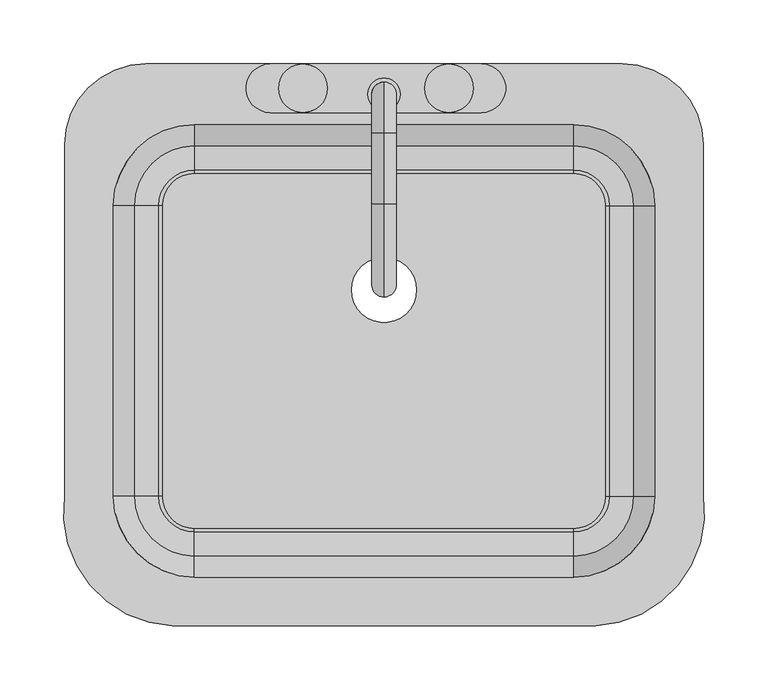
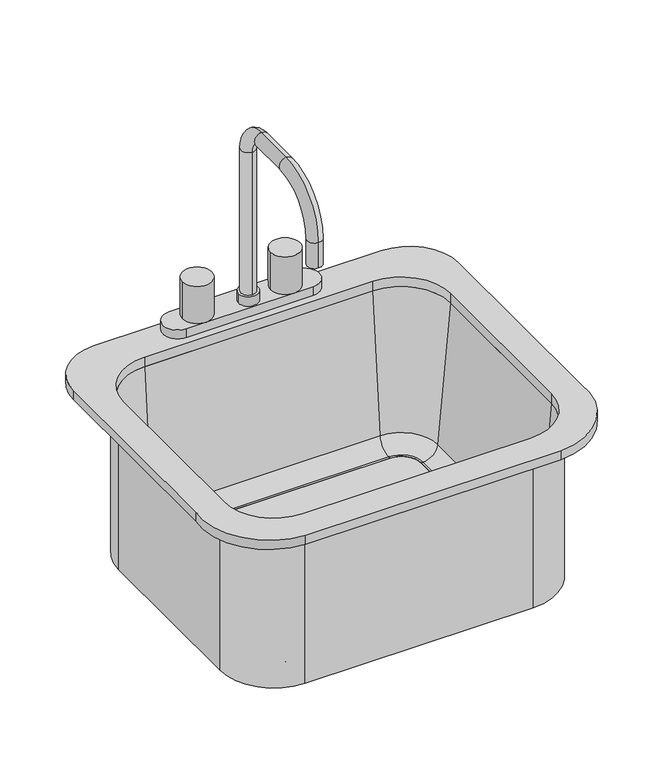
"""IFC4 building model written with IfcOpenShell, lengths in millimetres: flow terminal geometry."""

from ifc_helpers import new_model, si_unit, point, frame, frame_2d, origin, place, context, project, spatial, polyline, circle_curve, ellipse_curve, trimmed, segment, composite_curve, outline, extrude, source, transform, mapped, element, save
from ifc_brep_helpers import plane_surface, cylinder_surface, revolved_surface, advanced_brep


def flow_terminal_f629513f(model_context):
    return source(origin(), model_context, "Body", "SolidModel", [
        extrude(outline(composite_curve([segment(trimmed(circle_curve(frame_2d((-146.1534746, -170.8793432)), 89.0566732), [point((-149.9606923, -259.8545989))], [point((-234.3107593, -158.2545982))], False, "CARTESIAN"), True, "CONTINUOUS"), segment(polyline([(-234.3107593, -158.2545982), (-234.3107593, 116.6454011)]), True, "CONTINUOUS"), segment(trimmed(circle_curve(frame_2d((-170.8107593, 116.6454011)), 63.5), [point((-234.3107593, 116.6454011))], [point((-170.8107593, 180.1454011))], False, "CARTESIAN"), True, "CONTINUOUS"), segment(polyline([(-170.8107593, 180.1454011), (202.1892406, 180.1454011)]), True, "CONTINUOUS"), segment(trimmed(circle_curve(frame_2d((202.1892406, 116.6454011)), 63.5), [point((202.1892406, 180.1454011))], [point((265.6892406, 116.6454011))], False, "CARTESIAN"), True, "CONTINUOUS"), segment(polyline([(265.6892406, 116.6454011), (265.6892406, -158.2545989)]), True, "CONTINUOUS"), segment(trimmed(circle_curve(frame_2d((177.5319557, -170.8793432)), 89.0566732), [point((265.6892406, -158.2545989))], [point((181.3391735, -259.8545989))], False, "CARTESIAN"), True, "CONTINUOUS"), segment(polyline([(181.3391735, -259.8545989), (-149.9606923, -259.8545989)]), True, "CONTINUOUS")], self_intersect=False), holes=[composite_curve([segment(polyline([(164.0892406, 132.5204011), (-132.7107594, 132.5204011)]), True, "CONTINUOUS"), segment(trimmed(circle_curve(frame_2d((-132.7107594, 69.0204011)), 63.5), [point((-132.7107594, 132.5204011))], [point((-196.2107594, 69.0204011))], True, "CARTESIAN"), True, "CONTINUOUS"), segment(polyline([(-196.2107594, 69.0204011), (-196.2107594, -158.2545989)]), True, "CONTINUOUS"), segment(trimmed(circle_curve(frame_2d((-132.7107594, -158.2545989)), 63.5), [point((-196.2107594, -158.2545989))], [point((-132.7107594, -221.7545989))], True, "CARTESIAN"), True, "CONTINUOUS"), segment(polyline([(-132.7107594, -221.7545989), (164.0892406, -221.7545989)]), True, "CONTINUOUS"), segment(trimmed(circle_curve(frame_2d((164.0892406, -158.2545989)), 63.5), [point((164.0892406, -221.7545989))], [point((227.5892406, -158.2545989))], True, "CARTESIAN"), True, "CONTINUOUS"), segment(polyline([(227.5892406, -158.2545989), (227.5892406, 69.0204011)]), True, "CONTINUOUS"), segment(trimmed(circle_curve(frame_2d((164.0892406, 69.0204011)), 63.5), [point((227.5892406, 69.0204011))], [point((164.0892406, 132.5204011))], True, "CARTESIAN"), True, "CONTINUOUS")], self_intersect=False)]), frame((0.0, 0.0, 750.0), z_axis=(0.0, 0.0, 1.0), x_axis=(1.0, 0.0, 0.0)), (0.0, 0.0, 1.0), 12.7),
        advanced_brep(
        [(233.9392406, 69.0204011, 534.1), (164.0892406, 138.8704011, 534.1), (164.0892406, 138.8704011, 750.0), (233.9392406, 69.0204011, 750.0), (189.4892406, 69.0204011, 534.1), (164.0892406, 94.4204011, 534.1), (189.4892406, 69.0204011, 543.625), (164.0892406, 94.4204011, 543.625), (192.0776588, 69.0204011, 543.625), (164.0892406, 97.0088193, 543.625), (211.0551678, 69.0204011, 561.0146831), (164.0892406, 115.9863283, 561.0146831), (227.5892406, 69.0204011, 750.0), (164.0892406, 132.5204011, 750.0), (233.9392406, -158.2545989, 750.0), (233.9392406, -158.2545989, 534.1), (189.4892406, -158.2545989, 534.1), (189.4892406, -158.2545989, 543.625), (192.0776588, -158.2545989, 543.625), (211.0551678, -158.2545989, 561.0146831), (227.5892406, -158.2545989, 750.0), (164.0892406, -228.1045989, 534.1), (164.0892406, -228.1045989, 750.0), (164.0892406, -183.6545989, 534.1), (164.0892406, -183.6545989, 543.625), (164.0892406, -186.2430171, 543.625), (164.0892406, -205.2205261, 561.0146831), (164.0892406, -221.7545989, 750.0), (-132.7107594, -228.1045989, 750.0), (-132.7107594, -228.1045989, 534.1), (-132.7107594, -183.6545989, 534.1), (-132.7107594, -183.6545989, 543.625), (-132.7107594, -186.2430171, 543.625), (-132.7107594, -205.2205261, 561.0146831), (-132.7107594, -221.7545989, 750.0), (-202.5607594, -158.2545989, 534.1), (-202.5607594, -158.2545989, 750.0), (-158.1107594, -158.2545989, 534.1), (-158.1107594, -158.2545989, 543.625), (-160.6991776, -158.2545989, 543.625), (-179.6766866, -158.2545989, 561.0146831), (-196.2107594, -158.2545989, 750.0), (-202.5607594, 69.0204011, 750.0), (-202.5607594, 69.0204011, 534.1), (-158.1107594, 69.0204011, 534.1), (-158.1107594, 69.0204011, 543.625), (-160.6991776, 69.0204011, 543.625), (-179.6766866, 69.0204011, 561.0146831), (-196.2107594, 69.0204011, 750.0), (-132.7107594, 138.8704011, 534.1), (-132.7107594, 138.8704011, 750.0), (-132.7107594, 94.4204011, 534.1), (-132.7107594, 94.4204011, 543.625), (-132.7107594, 97.0088193, 543.625), (-132.7107594, 115.9863283, 561.0146831), (-132.7107594, 132.5204011, 750.0)],
        [
            (0, 1, circle_curve(frame((164.0892406, 69.0204011, 534.1), z_axis=(0.0, 0.0, 1.0), x_axis=(0.0, 1.0, 0.0)), 69.85)),
            (1, 2),
            (2, 3, circle_curve(frame((164.0892406, 69.0204011, 750.0), z_axis=(0.0, 0.0, -1.0), x_axis=(0.0, 1.0, 0.0)), 69.85)),
            (3, 0),
            (4, 5, circle_curve(frame((164.0892406, 69.0204011, 534.1), z_axis=(0.0, 0.0, 1.0), x_axis=(0.0, 1.0, 0.0)), 25.4)),
            (5, 1),
            (0, 4),
            (6, 7, circle_curve(frame((164.0892406, 69.0204011, 543.625), z_axis=(0.0, 0.0, 1.0), x_axis=(0.0, 1.0, 0.0)), 25.4)),
            (7, 5),
            (4, 6),
            (8, 9, circle_curve(frame((164.0892406, 69.0204011, 543.625), z_axis=(0.0, 0.0, 1.0), x_axis=(0.0, 1.0, 0.0)), 27.9884182)),
            (9, 7),
            (6, 8),
            (10, 11, circle_curve(frame((164.0892406, 69.0204011, 561.0146831), z_axis=(0.0, 0.0, 1.0), x_axis=(0.0, 1.0, 0.0)), 46.9659272)),
            (11, 9, circle_curve(frame((164.0892406, 97.0088193, 562.675), z_axis=(-1.0, 0.0, 0.0), x_axis=(0.0, 1.0, 0.0)), 19.05)),
            (8, 10, circle_curve(frame((192.0776588, 69.0204011, 562.675), z_axis=(0.0, -1.0, 0.0), x_axis=(1.0, 0.0, 0.0)), 19.05)),
            (12, 13, circle_curve(frame((164.0892406, 69.0204011, 750.0), z_axis=(0.0, 0.0, 1.0), x_axis=(0.0, 1.0, 0.0)), 63.5)),
            (13, 11),
            (10, 12),
            (2, 13),
            (12, 3),
            (3, 14),
            (14, 15),
            (15, 0),
            (15, 16),
            (16, 4),
            (16, 17),
            (17, 6),
            (17, 18),
            (18, 8),
            (18, 19, circle_curve(frame((192.0776588, -158.2545989, 562.675), z_axis=(0.0, -1.0, 0.0), x_axis=(1.0, 0.0, 0.0)), 19.05)),
            (19, 10),
            (19, 20),
            (20, 12),
            (20, 14),
            (21, 15, circle_curve(frame((164.0892406, -158.2545989, 534.1), z_axis=(0.0, 0.0, 1.0), x_axis=(1.0, 0.0, 0.0)), 69.85)),
            (14, 22, circle_curve(frame((164.0892406, -158.2545989, 750.0), z_axis=(0.0, 0.0, -1.0), x_axis=(1.0, 0.0, 0.0)), 69.85)),
            (22, 21),
            (23, 16, circle_curve(frame((164.0892406, -158.2545989, 534.1), z_axis=(0.0, 0.0, 1.0), x_axis=(1.0, 0.0, 0.0)), 25.4)),
            (21, 23),
            (24, 17, circle_curve(frame((164.0892406, -158.2545989, 543.625), z_axis=(0.0, 0.0, 1.0), x_axis=(1.0, 0.0, 0.0)), 25.4)),
            (23, 24),
            (25, 18, circle_curve(frame((164.0892406, -158.2545989, 543.625), z_axis=(0.0, 0.0, 1.0), x_axis=(1.0, 0.0, 0.0)), 27.9884182)),
            (24, 25),
            (26, 19, circle_curve(frame((164.0892406, -158.2545989, 561.0146831), z_axis=(0.0, 0.0, 1.0), x_axis=(1.0, 0.0, 0.0)), 46.9659272)),
            (25, 26, circle_curve(frame((164.0892406, -186.2430171, 562.675), z_axis=(-1.0, 0.0, 0.0), x_axis=(0.0, -1.0, 0.0)), 19.05)),
            (27, 20, circle_curve(frame((164.0892406, -158.2545989, 750.0), z_axis=(0.0, 0.0, 1.0), x_axis=(1.0, 0.0, 0.0)), 63.5)),
            (26, 27),
            (27, 22),
            (22, 28),
            (28, 29),
            (29, 21),
            (29, 30),
            (30, 23),
            (30, 31),
            (31, 24),
            (31, 32),
            (32, 25),
            (32, 33, circle_curve(frame((-132.7107594, -186.2430171, 562.675), z_axis=(-1.0, 0.0, 0.0), x_axis=(0.0, -1.0, 0.0)), 19.05)),
            (33, 26),
            (33, 34),
            (34, 27),
            (34, 28),
            (35, 29, circle_curve(frame((-132.7107594, -158.2545989, 534.1), z_axis=(0.0, 0.0, 1.0), x_axis=(0.0, -1.0, 0.0)), 69.85)),
            (28, 36, circle_curve(frame((-132.7107594, -158.2545989, 750.0), z_axis=(0.0, 0.0, -1.0), x_axis=(0.0, -1.0, 0.0)), 69.85)),
            (36, 35),
            (37, 30, circle_curve(frame((-132.7107594, -158.2545989, 534.1), z_axis=(0.0, 0.0, 1.0), x_axis=(0.0, -1.0, 0.0)), 25.4)),
            (35, 37),
            (38, 31, circle_curve(frame((-132.7107594, -158.2545989, 543.625), z_axis=(0.0, 0.0, 1.0), x_axis=(0.0, -1.0, 0.0)), 25.4)),
            (37, 38),
            (39, 32, circle_curve(frame((-132.7107594, -158.2545989, 543.625), z_axis=(0.0, 0.0, 1.0), x_axis=(0.0, -1.0, 0.0)), 27.9884182)),
            (38, 39),
            (40, 33, circle_curve(frame((-132.7107594, -158.2545989, 561.0146831), z_axis=(0.0, 0.0, 1.0), x_axis=(0.0, -1.0, 0.0)), 46.9659272)),
            (39, 40, circle_curve(frame((-160.6991776, -158.2545989, 562.675), z_axis=(0.0, 1.0, 0.0), x_axis=(-1.0, 0.0, 0.0)), 19.05)),
            (41, 34, circle_curve(frame((-132.7107594, -158.2545989, 750.0), z_axis=(0.0, 0.0, 1.0), x_axis=(0.0, -1.0, 0.0)), 63.5)),
            (40, 41),
            (41, 36),
            (36, 42),
            (42, 43),
            (43, 35),
            (43, 44),
            (44, 37),
            (44, 45),
            (45, 38),
            (45, 46),
            (46, 39),
            (46, 47, circle_curve(frame((-160.6991776, 69.0204011, 562.675), z_axis=(0.0, 1.0, 0.0), x_axis=(-1.0, 0.0, 0.0)), 19.05)),
            (47, 40),
            (47, 48),
            (48, 41),
            (48, 42),
            (49, 43, circle_curve(frame((-132.7107594, 69.0204011, 534.1), z_axis=(0.0, 0.0, 1.0), x_axis=(-1.0, 0.0, 0.0)), 69.85)),
            (42, 50, circle_curve(frame((-132.7107594, 69.0204011, 750.0), z_axis=(0.0, 0.0, -1.0), x_axis=(-1.0, 0.0, 0.0)), 69.85)),
            (50, 49),
            (51, 44, circle_curve(frame((-132.7107594, 69.0204011, 534.1), z_axis=(0.0, 0.0, 1.0), x_axis=(-1.0, 0.0, 0.0)), 25.4)),
            (49, 51),
            (52, 45, circle_curve(frame((-132.7107594, 69.0204011, 543.625), z_axis=(0.0, 0.0, 1.0), x_axis=(-1.0, 0.0, 0.0)), 25.4)),
            (51, 52),
            (53, 46, circle_curve(frame((-132.7107594, 69.0204011, 543.625), z_axis=(0.0, 0.0, 1.0), x_axis=(-1.0, 0.0, 0.0)), 27.9884182)),
            (52, 53),
            (54, 47, circle_curve(frame((-132.7107594, 69.0204011, 561.0146831), z_axis=(0.0, 0.0, 1.0), x_axis=(-1.0, 0.0, 0.0)), 46.9659272)),
            (53, 54, circle_curve(frame((-132.7107594, 97.0088193, 562.675), z_axis=(1.0, 0.0, 0.0), x_axis=(0.0, 1.0, 0.0)), 19.05)),
            (55, 48, circle_curve(frame((-132.7107594, 69.0204011, 750.0), z_axis=(0.0, 0.0, 1.0), x_axis=(-1.0, 0.0, 0.0)), 63.5)),
            (54, 55),
            (55, 50),
            (50, 2),
            (1, 49),
            (5, 51),
            (7, 52),
            (9, 53),
            (11, 54),
            (13, 55),
        ],
        [
            cylinder_surface(frame((164.0892406, 69.0204011, 0.0), z_axis=(0.0, 0.0, -1.0), x_axis=(0.0, 1.0, 0.0)), 69.85),
            plane_surface(frame((164.0892406, 69.0204011, 534.1), z_axis=(0.0, 0.0, -1.0), x_axis=(0.0, 1.0, 0.0))),
            revolved_surface(polyline([(164.0892406, 94.42040109999999, 534.1), (164.0892406, 94.42040109999999, 543.625)]), (164.0892406, 69.0204011, 0.0), (0.0, 0.0, -1.0)),
            plane_surface(frame((164.0892406, 69.0204011, 543.625), z_axis=(0.0, 0.0, 1.0), x_axis=(0.0, 1.0, 0.0))),
            revolved_surface(trimmed(ellipse_curve(frame((164.0892406, 97.0088193, 562.675), z_axis=(1.0, 0.0, 0.0), x_axis=(0.0, 1.0, 0.0)), 19.05, 19.05), [point((164.0892406, 97.0088193, 543.625))], [point((164.0892406, 115.9863283, 561.0146831))], True, "CARTESIAN"), (164.0892406, 69.0204011, 0.0), (0.0, 0.0, -1.0)),
            revolved_surface(polyline([(164.0892406, 115.9863283, 561.0146831), (164.0892406, 132.5204011, 750.0)]), (164.0892406, 69.0204011, 0.0), (0.0, 0.0, -1.0)),
            plane_surface(frame((164.0892406, 69.0204011, 750.0), z_axis=(0.0, 0.0, 1.0), x_axis=(0.0, 1.0, 0.0))),
            plane_surface(frame((233.9392406, 69.0204011, 750.0), z_axis=(1.0, 0.0, 0.0), x_axis=(0.0, -1.0, 0.0))),
            plane_surface(frame((233.9392406, 69.0204011, 534.1), z_axis=(0.0, 0.0, -1.0), x_axis=(0.0, -1.0, 0.0))),
            plane_surface(frame((189.4892406, 69.0204011, 534.1), z_axis=(-1.0, 0.0, 0.0), x_axis=(0.0, -1.0, 0.0))),
            plane_surface(frame((189.4892406, 69.0204011, 543.625), z_axis=(0.0, 0.0, 1.0), x_axis=(0.0, -1.0, 0.0))),
            revolved_surface(polyline([(211.1276588, -158.25459889999996, 562.675), (211.1276588, 69.0204011, 562.675)]), (192.0776588, 69.0204011, 562.675), (0.0, -1.0, 0.0)),
            plane_surface(frame((211.0551678, 69.0204011, 561.0146831), z_axis=(-0.9961946980917442, 0.0, 0.0871557427476735), x_axis=(0.0, -1.0, 0.0))),
            plane_surface(frame((227.5892406, 69.0204011, 750.0), z_axis=(0.0, 0.0, 1.0), x_axis=(0.0, -1.0, 0.0))),
            cylinder_surface(frame((164.0892406, -158.2545989, 0.0), z_axis=(0.0, 0.0, -1.0), x_axis=(1.0, 0.0, 0.0)), 69.85),
            plane_surface(frame((164.0892406, -158.2545989, 534.1), z_axis=(0.0, 0.0, -1.0), x_axis=(1.0, 0.0, 0.0))),
            revolved_surface(polyline([(189.48924060000002, -158.2545989, 534.1), (189.48924060000002, -158.2545989, 543.625)]), (164.0892406, -158.2545989, 0.0), (0.0, 0.0, -1.0)),
            plane_surface(frame((164.0892406, -158.2545989, 543.625), z_axis=(0.0, 0.0, 1.0), x_axis=(1.0, 0.0, 0.0))),
            revolved_surface(trimmed(ellipse_curve(frame((192.0776588, -158.2545989, 562.675), z_axis=(0.0, -1.0, 0.0), x_axis=(1.0, 0.0, 0.0)), 19.05, 19.05), [point((192.0776588, -158.2545989, 543.625))], [point((211.0551678, -158.2545989, 561.0146831))], True, "CARTESIAN"), (164.0892406, -158.2545989, 0.0), (0.0, 0.0, -1.0)),
            revolved_surface(polyline([(211.0551678, -158.2545989, 561.0146831), (227.5892406, -158.2545989, 750.0)]), (164.0892406, -158.2545989, 0.0), (0.0, 0.0, -1.0)),
            plane_surface(frame((164.0892406, -158.2545989, 750.0), z_axis=(0.0, 0.0, 1.0), x_axis=(1.0, 0.0, 0.0))),
            plane_surface(frame((164.0892406, -228.1045989, 750.0), z_axis=(0.0, -1.0, 0.0), x_axis=(-1.0, 0.0, 0.0))),
            plane_surface(frame((164.0892406, -228.1045989, 534.1), z_axis=(0.0, 0.0, -1.0), x_axis=(-1.0, 0.0, 0.0))),
            plane_surface(frame((164.0892406, -183.6545989, 534.1), z_axis=(0.0, 1.0, 0.0), x_axis=(-1.0, 0.0, 0.0))),
            plane_surface(frame((164.0892406, -183.6545989, 543.625), z_axis=(0.0, 0.0, 1.0), x_axis=(-1.0, 0.0, 0.0))),
            revolved_surface(polyline([(-132.7107594, -205.29301710000001, 562.675), (164.0892406, -205.29301710000001, 562.675)]), (164.0892406, -186.2430171, 562.675), (-1.0, 0.0, 0.0)),
            plane_surface(frame((164.0892406, -205.2205261, 561.0146831), z_axis=(0.0, 0.9961946980917442, 0.0871557427476735), x_axis=(-1.0, 0.0, 0.0))),
            plane_surface(frame((164.0892406, -221.7545989, 750.0), z_axis=(0.0, 0.0, 1.0), x_axis=(-1.0, 0.0, 0.0))),
            cylinder_surface(frame((-132.7107594, -158.2545989, 0.0), z_axis=(0.0, 0.0, -1.0), x_axis=(0.0, -1.0, 0.0)), 69.85),
            plane_surface(frame((-132.7107594, -158.2545989, 534.1), z_axis=(0.0, 0.0, -1.0), x_axis=(0.0, -1.0, 0.0))),
            revolved_surface(polyline([(-132.7107594, -183.6545989, 534.1), (-132.7107594, -183.6545989, 543.625)]), (-132.7107594, -158.2545989, 0.0), (0.0, 0.0, -1.0)),
            plane_surface(frame((-132.7107594, -158.2545989, 543.625), z_axis=(0.0, 0.0, 1.0), x_axis=(0.0, -1.0, 0.0))),
            revolved_surface(trimmed(ellipse_curve(frame((-132.7107594, -186.2430171, 562.675), z_axis=(-1.0, 0.0, 0.0), x_axis=(0.0, -1.0, 0.0)), 19.05, 19.05), [point((-132.7107594, -186.2430171, 543.625))], [point((-132.7107594, -205.2205261, 561.0146831))], True, "CARTESIAN"), (-132.7107594, -158.2545989, 0.0), (0.0, 0.0, -1.0)),
            revolved_surface(polyline([(-132.7107594, -205.2205261, 561.0146831), (-132.7107594, -221.7545989, 750.0)]), (-132.7107594, -158.2545989, 0.0), (0.0, 0.0, -1.0)),
            plane_surface(frame((-132.7107594, -158.2545989, 750.0), z_axis=(0.0, 0.0, 1.0), x_axis=(0.0, -1.0, 0.0))),
            plane_surface(frame((-202.5607594, -158.2545989, 750.0), z_axis=(-1.0, 0.0, 0.0), x_axis=(0.0, 1.0, 0.0))),
            plane_surface(frame((-202.5607594, -158.2545989, 534.1), z_axis=(0.0, 0.0, -1.0), x_axis=(0.0, 1.0, 0.0))),
            plane_surface(frame((-158.1107594, -158.2545989, 534.1), z_axis=(1.0, 0.0, 0.0), x_axis=(0.0, 1.0, 0.0))),
            plane_surface(frame((-158.1107594, -158.2545989, 543.625), z_axis=(0.0, 0.0, 1.0), x_axis=(0.0, 1.0, 0.0))),
            revolved_surface(polyline([(-179.74917760000002, 69.02040109999999, 562.675), (-179.74917760000002, -158.2545989, 562.675)]), (-160.6991776, -158.2545989, 562.675), (0.0, 1.0, 0.0)),
            plane_surface(frame((-179.6766866, -158.2545989, 561.0146831), z_axis=(0.9961946980917442, 0.0, 0.0871557427476735), x_axis=(0.0, 1.0, 0.0))),
            plane_surface(frame((-196.2107594, -158.2545989, 750.0), z_axis=(0.0, 0.0, 1.0), x_axis=(0.0, 1.0, 0.0))),
            cylinder_surface(frame((-132.7107594, 69.0204011, 0.0), z_axis=(0.0, 0.0, -1.0), x_axis=(-1.0, 0.0, 0.0)), 69.85),
            plane_surface(frame((-132.7107594, 69.0204011, 534.1), z_axis=(0.0, 0.0, -1.0), x_axis=(-1.0, 0.0, 0.0))),
            revolved_surface(polyline([(-158.1107594, 69.0204011, 534.1), (-158.1107594, 69.0204011, 543.625)]), (-132.7107594, 69.0204011, 0.0), (0.0, 0.0, -1.0)),
            plane_surface(frame((-132.7107594, 69.0204011, 543.625), z_axis=(0.0, 0.0, 1.0), x_axis=(-1.0, 0.0, 0.0))),
            revolved_surface(trimmed(ellipse_curve(frame((-160.6991776, 69.0204011, 562.675), z_axis=(0.0, 1.0, 0.0), x_axis=(-1.0, 0.0, 0.0)), 19.05, 19.05), [point((-160.6991776, 69.0204011, 543.625))], [point((-179.6766866, 69.0204011, 561.0146831))], True, "CARTESIAN"), (-132.7107594, 69.0204011, 0.0), (0.0, 0.0, -1.0)),
            revolved_surface(polyline([(-179.6766866, 69.0204011, 561.0146831), (-196.2107594, 69.0204011, 750.0)]), (-132.7107594, 69.0204011, 0.0), (0.0, 0.0, -1.0)),
            plane_surface(frame((-132.7107594, 69.0204011, 750.0), z_axis=(0.0, 0.0, 1.0), x_axis=(-1.0, 0.0, 0.0))),
            plane_surface(frame((-132.7107594, 138.8704011, 750.0), z_axis=(0.0, 1.0, 0.0), x_axis=(1.0, 0.0, 0.0))),
            plane_surface(frame((-132.7107594, 138.8704011, 534.1), z_axis=(0.0, 0.0, -1.0), x_axis=(1.0, 0.0, 0.0))),
            plane_surface(frame((-132.7107594, 94.4204011, 534.1), z_axis=(0.0, -1.0, 0.0), x_axis=(1.0, 0.0, 0.0))),
            plane_surface(frame((-132.7107594, 94.4204011, 543.625), z_axis=(0.0, 0.0, 1.0), x_axis=(1.0, 0.0, 0.0))),
            revolved_surface(polyline([(164.0892406, 116.0588193, 562.675), (-132.7107594, 116.0588193, 562.675)]), (-132.7107594, 97.0088193, 562.675), (1.0, 0.0, 0.0)),
            plane_surface(frame((-132.7107594, 115.9863283, 561.0146831), z_axis=(0.0, -0.9961946980917442, 0.0871557427476735), x_axis=(1.0, 0.0, 0.0))),
            plane_surface(frame((-132.7107594, 132.5204011, 750.0), z_axis=(0.0, 0.0, 1.0), x_axis=(1.0, 0.0, 0.0))),
        ],
        [
            (0, [[1, 2, 3, 4]]),
            (1, [[5, 6, -1, 7]]),
            (2, [[8, 9, -5, 10]]),
            (3, [[11, 12, -8, 13]]),
            (4, [[14, 15, -11, 16]]),
            (5, [[17, 18, -14, 19]]),
            (6, [[-3, 20, -17, 21]]),
            (7, [[-4, 22, 23, 24]]),
            (8, [[-7, -24, 25, 26]]),
            (9, [[-10, -26, 27, 28]]),
            (10, [[-13, -28, 29, 30]]),
            (11, [[-16, -30, 31, 32]]),
            (12, [[-19, -32, 33, 34]]),
            (13, [[-21, -34, 35, -22]]),
            (14, [[36, -23, 37, 38]]),
            (15, [[39, -25, -36, 40]]),
            (16, [[41, -27, -39, 42]]),
            (17, [[43, -29, -41, 44]]),
            (18, [[45, -31, -43, 46]]),
            (19, [[47, -33, -45, 48]]),
            (20, [[-37, -35, -47, 49]]),
            (21, [[-38, 50, 51, 52]]),
            (22, [[-40, -52, 53, 54]]),
            (23, [[-42, -54, 55, 56]]),
            (24, [[-44, -56, 57, 58]]),
            (25, [[-46, -58, 59, 60]]),
            (26, [[-48, -60, 61, 62]]),
            (27, [[-49, -62, 63, -50]]),
            (28, [[64, -51, 65, 66]]),
            (29, [[67, -53, -64, 68]]),
            (30, [[69, -55, -67, 70]]),
            (31, [[71, -57, -69, 72]]),
            (32, [[73, -59, -71, 74]]),
            (33, [[75, -61, -73, 76]]),
            (34, [[-65, -63, -75, 77]]),
            (35, [[-66, 78, 79, 80]]),
            (36, [[-68, -80, 81, 82]]),
            (37, [[-70, -82, 83, 84]]),
            (38, [[-72, -84, 85, 86]]),
            (39, [[-74, -86, 87, 88]]),
            (40, [[-76, -88, 89, 90]]),
            (41, [[-77, -90, 91, -78]]),
            (42, [[92, -79, 93, 94]]),
            (43, [[95, -81, -92, 96]]),
            (44, [[97, -83, -95, 98]]),
            (45, [[99, -85, -97, 100]]),
            (46, [[101, -87, -99, 102]]),
            (47, [[103, -89, -101, 104]]),
            (48, [[-93, -91, -103, 105]]),
            (49, [[-94, 106, -2, 107]]),
            (50, [[-96, -107, -6, 108]]),
            (51, [[-98, -108, -9, 109]]),
            (52, [[-100, -109, -12, 110]]),
            (53, [[-102, -110, -15, 111]]),
            (54, [[-104, -111, -18, 112]]),
            (55, [[-105, -112, -20, -106]]),
        ],
    ),
        extrude(outline(composite_curve([segment(trimmed(circle_curve(frame_2d((164.0892406, 69.0204011)), 25.4), [point((164.0892406, 94.4204011))], [point((189.4892406, 69.0204011))], False, "CARTESIAN"), True, "CONTINUOUS"), segment(polyline([(189.4892406, 69.0204011), (189.4892406, -158.2545989)]), True, "CONTINUOUS"), segment(trimmed(circle_curve(frame_2d((164.0892406, -158.2545989)), 25.4), [point((189.4892406, -158.2545989))], [point((164.0892406, -183.6545989))], False, "CARTESIAN"), True, "CONTINUOUS"), segment(polyline([(164.0892406, -183.6545989), (-132.7107594, -183.6545989)]), True, "CONTINUOUS"), segment(trimmed(circle_curve(frame_2d((-132.7107594, -158.2545989)), 25.4), [point((-132.7107594, -183.6545989))], [point((-158.1107594, -158.2545989))], False, "CARTESIAN"), True, "CONTINUOUS"), segment(polyline([(-158.1107594, -158.2545989), (-158.1107594, 69.0204011)]), True, "CONTINUOUS"), segment(trimmed(circle_curve(frame_2d((-132.7107594, 69.0204011)), 25.4), [point((-158.1107594, 69.0204011))], [point((-132.7107594, 94.4204011))], False, "CARTESIAN"), True, "CONTINUOUS"), segment(polyline([(-132.7107594, 94.4204011), (164.0892406, 94.4204011)]), True, "CONTINUOUS")], self_intersect=False), holes=[composite_curve([segment(trimmed(circle_curve(frame_2d((15.6892406, 3.175)), 25.4), [point((-9.7107594, 3.175))], [point((41.0892406, 3.175))], True, "CARTESIAN"), True, "CONTINUOUS"), segment(trimmed(circle_curve(frame_2d((15.6892406, 3.175)), 25.4), [point((41.0892406, 3.175))], [point((-9.7107594, 3.175))], True, "CARTESIAN"), True, "CONTINUOUS")], self_intersect=False)]), frame((0.0, 0.0, 534.1), z_axis=(0.0, 0.0, 1.0), x_axis=(1.0, 0.0, 0.0)), (0.0, 0.0, 1.0), 9.525),
        advanced_brep(
        [(-66.8607594, 161.0954011, 826.2), (-28.7607594, 161.0954011, 826.2), (47.4392406, 161.0954011, 826.2), (85.5392406, 161.0954011, 826.2), (91.8892406, 180.1454011, 762.7), (91.8892406, 142.0454011, 762.7), (-73.2107594, 142.0454011, 762.7), (-73.2107594, 180.1454011, 762.7), (-66.8607594, 161.0954011, 775.2), (-47.8107594, 142.0454011, 775.2), (-28.7607594, 161.0954011, 775.2), (-47.8107594, 180.1454011, 775.2), (47.4392406, 161.0954011, 775.2), (66.4892406, 142.0454011, 775.2), (85.5392406, 161.0954011, 775.2), (66.4892406, 180.1454011, 775.2), (-73.2107594, 180.1454011, 775.2), (-73.2107594, 142.0454011, 775.2), (91.8892406, 142.0454011, 775.2), (91.8892406, 180.1454011, 775.2), (28.3892406, 156.3329011, 775.2), (2.9892406, 156.3329011, 775.2), (15.6892406, 165.8579011, 983.3625), (15.6892406, 146.8079011, 983.3625), (15.6892406, 146.8079011, 788.1), (15.6892406, 165.8579011, 788.1), (15.6892406, 126.1704011, 1023.05), (15.6892406, 126.1704011, 1004.0), (15.6892406, 70.6079011, 1023.05), (15.6892406, 70.6079011, 1004.0), (15.6892406, -2.4170989, 950.025), (15.6892406, 16.6329011, 950.025), (15.6892406, -2.4170989, 915.1), (15.6892406, 16.6329011, 915.1), (2.9892406, 156.3329011, 788.1), (28.3892406, 156.3329011, 788.1)],
        [
            (0, 1, circle_curve(frame((-47.8107594, 161.0954011, 826.2), z_axis=(0.0, 0.0, 1.0), x_axis=(1.0, 0.0, 0.0)), 19.05)),
            (1, 0, circle_curve(frame((-47.8107594, 161.0954011, 826.2), z_axis=(0.0, 0.0, 1.0), x_axis=(1.0, 0.0, 0.0)), 19.05)),
            (2, 3, circle_curve(frame((66.4892406, 161.0954011, 826.2), z_axis=(0.0, 0.0, 1.0), x_axis=(1.0, 0.0, 0.0)), 19.05)),
            (3, 2, circle_curve(frame((66.4892406, 161.0954011, 826.2), z_axis=(0.0, 0.0, 1.0), x_axis=(1.0, 0.0, 0.0)), 19.05)),
            (4, 5, circle_curve(frame((91.8892406, 161.0954011, 762.7), z_axis=(0.0, 0.0, -1.0), x_axis=(1.0, 0.0, 0.0)), 19.05)),
            (5, 6),
            (6, 7, circle_curve(frame((-73.2107594, 161.0954011, 762.7), z_axis=(0.0, 0.0, -1.0), x_axis=(1.0, 0.0, 0.0)), 19.05)),
            (7, 4),
            (0, 8),
            (8, 9, circle_curve(frame((-47.8107594, 161.0954011, 775.2), z_axis=(0.0, 0.0, 1.0), x_axis=(1.0, 0.0, 0.0)), 19.05)),
            (9, 10, circle_curve(frame((-47.8107594, 161.0954011, 775.2), z_axis=(0.0, 0.0, 1.0), x_axis=(1.0, 0.0, 0.0)), 19.05)),
            (10, 1),
            (10, 11, circle_curve(frame((-47.8107594, 161.0954011, 775.2), z_axis=(0.0, 0.0, 1.0), x_axis=(1.0, 0.0, 0.0)), 19.05)),
            (11, 8, circle_curve(frame((-47.8107594, 161.0954011, 775.2), z_axis=(0.0, 0.0, 1.0), x_axis=(1.0, 0.0, 0.0)), 19.05)),
            (2, 12),
            (12, 13, circle_curve(frame((66.4892406, 161.0954011, 775.2), z_axis=(0.0, 0.0, 1.0), x_axis=(1.0, 0.0, 0.0)), 19.05)),
            (13, 14, circle_curve(frame((66.4892406, 161.0954011, 775.2), z_axis=(0.0, 0.0, 1.0), x_axis=(1.0, 0.0, 0.0)), 19.05)),
            (14, 3),
            (14, 15, circle_curve(frame((66.4892406, 161.0954011, 775.2), z_axis=(0.0, 0.0, 1.0), x_axis=(1.0, 0.0, 0.0)), 19.05)),
            (15, 12, circle_curve(frame((66.4892406, 161.0954011, 775.2), z_axis=(0.0, 0.0, 1.0), x_axis=(1.0, 0.0, 0.0)), 19.05)),
            (16, 17, circle_curve(frame((-73.2107594, 161.0954011, 775.2), z_axis=(0.0, 0.0, 1.0), x_axis=(1.0, 0.0, 0.0)), 19.05)),
            (17, 9),
            (11, 16),
            (18, 19, circle_curve(frame((91.8892406, 161.0954011, 775.2), z_axis=(0.0, 0.0, 1.0), x_axis=(1.0, 0.0, 0.0)), 19.05)),
            (19, 15),
            (13, 18),
            (15, 11),
            (9, 13),
            (20, 21, circle_curve(frame((15.6892406, 156.3329011, 775.2), z_axis=(0.0, 0.0, -1.0), x_axis=(1.0, 0.0, 0.0)), 12.7)),
            (21, 20, circle_curve(frame((15.6892406, 156.3329011, 775.2), z_axis=(0.0, 0.0, -1.0), x_axis=(1.0, 0.0, 0.0)), 12.7)),
            (19, 4),
            (7, 16),
            (6, 17),
            (5, 18),
            (22, 23, circle_curve(frame((15.6892406, 156.3329011, 983.3625), z_axis=(0.0, 0.0, -1.0), x_axis=(0.0, -1.0, 0.0)), 9.525)),
            (23, 24),
            (24, 25, circle_curve(frame((15.6892406, 156.3329011, 788.1), z_axis=(0.0, 0.0, 1.0), x_axis=(0.0, -1.0, 0.0)), 9.525)),
            (25, 22),
            (23, 22, circle_curve(frame((15.6892406, 156.3329011, 983.3625), z_axis=(0.0, 0.0, -1.0), x_axis=(0.0, -1.0, 0.0)), 9.525)),
            (25, 24, circle_curve(frame((15.6892406, 156.3329011, 788.1), z_axis=(0.0, 0.0, 1.0), x_axis=(0.0, -1.0, 0.0)), 9.525)),
            (22, 26, circle_curve(frame((15.6892406, 126.1704011, 983.3625), z_axis=(1.0, 0.0, 0.0), x_axis=(0.0, 1.0, 0.0)), 39.6875)),
            (26, 27, circle_curve(frame((15.6892406, 126.1704011, 1013.525), z_axis=(0.0, 1.0, 0.0), x_axis=(0.0, 0.0, -1.0)), 9.525)),
            (27, 23, circle_curve(frame((15.6892406, 126.1704011, 983.3625), z_axis=(-1.0, 0.0, 0.0), x_axis=(0.0, 1.0, 0.0)), 20.6375)),
            (27, 26, circle_curve(frame((15.6892406, 126.1704011, 1013.525), z_axis=(0.0, 1.0, 0.0), x_axis=(0.0, 0.0, -1.0)), 9.525)),
            (26, 28),
            (28, 29, circle_curve(frame((15.6892406, 70.6079011, 1013.525), z_axis=(0.0, 1.0, 0.0), x_axis=(0.0, 0.0, -1.0)), 9.525)),
            (29, 27),
            (29, 28, circle_curve(frame((15.6892406, 70.6079011, 1013.525), z_axis=(0.0, 1.0, 0.0), x_axis=(0.0, 0.0, -1.0)), 9.525)),
            (28, 30, circle_curve(frame((15.6892406, 70.6079011, 950.025), z_axis=(1.0, 0.0, 0.0), x_axis=(0.0, 0.0, 1.0)), 73.025)),
            (30, 31, circle_curve(frame((15.6892406, 7.1079011, 950.025), z_axis=(0.0, 0.0, 1.0), x_axis=(0.0, 1.0, 0.0)), 9.525)),
            (31, 29, circle_curve(frame((15.6892406, 70.6079011, 950.025), z_axis=(-1.0, 0.0, 0.0), x_axis=(0.0, 0.0, 1.0)), 53.975)),
            (31, 30, circle_curve(frame((15.6892406, 7.1079011, 950.025), z_axis=(0.0, 0.0, 1.0), x_axis=(0.0, 1.0, 0.0)), 9.525)),
            (32, 33, circle_curve(frame((15.6892406, 7.1079011, 915.1), z_axis=(0.0, 0.0, -1.0), x_axis=(0.0, 1.0, 0.0)), 9.525)),
            (33, 32, circle_curve(frame((15.6892406, 7.1079011, 915.1), z_axis=(0.0, 0.0, -1.0), x_axis=(0.0, 1.0, 0.0)), 9.525)),
            (30, 32),
            (33, 31),
            (34, 35, circle_curve(frame((15.6892406, 156.3329011, 788.1), z_axis=(0.0, 0.0, 1.0), x_axis=(1.0, 0.0, 0.0)), 12.7)),
            (35, 34, circle_curve(frame((15.6892406, 156.3329011, 788.1), z_axis=(0.0, 0.0, 1.0), x_axis=(1.0, 0.0, 0.0)), 12.7)),
            (34, 21),
            (20, 35),
        ],
        [
            plane_surface(frame((-28.7607594, 161.0954011, 826.2), z_axis=(0.0, 0.0, 1.0), x_axis=(0.0, 1.0, 0.0))),
            plane_surface(frame((-28.7607594, 161.0954011, 762.7), z_axis=(0.0, 0.0, -1.0), x_axis=(0.0, -1.0, 0.0))),
            cylinder_surface(frame((-47.8107594, 161.0954011, 762.7), z_axis=(0.0, 0.0, 1.0), x_axis=(1.0, 0.0, 0.0)), 19.05),
            cylinder_surface(frame((66.4892406, 161.0954011, 0.0), z_axis=(0.0, 0.0, 1.0), x_axis=(1.0, 0.0, 0.0)), 19.05),
            plane_surface(frame((-73.2107594, 180.1454011, 775.2), z_axis=(0.0, 0.0, 1.0), x_axis=(-1.0, 0.0, 0.0))),
            plane_surface(frame((91.8892406, 180.1454011, 775.2), z_axis=(0.0, 1.0, 0.0), x_axis=(0.0, 0.0, -1.0))),
            cylinder_surface(frame((-73.2107594, 161.0954011, 762.7), z_axis=(0.0, 0.0, 1.0), x_axis=(1.0, 0.0, 0.0)), 19.05),
            plane_surface(frame((-73.2107594, 142.0454011, 775.2), z_axis=(0.0, -1.0, 0.0), x_axis=(0.0, 0.0, -1.0))),
            cylinder_surface(frame((91.8892406, 161.0954011, 762.7), z_axis=(0.0, 0.0, 1.0), x_axis=(1.0, 0.0, 0.0)), 19.05),
            cylinder_surface(frame((15.6892406, 156.3329011, 762.7), z_axis=(0.0, 0.0, -1.0), x_axis=(0.0, -1.0, 0.0)), 9.525),
            revolved_surface(trimmed(ellipse_curve(frame((15.6892406, 156.3329011, 983.3625), z_axis=(0.0, 0.0, -1.0), x_axis=(0.0, -1.0, 0.0)), 9.525, 9.525), [point((15.6892406, 165.8579011, 983.3625))], [point((15.6892406, 146.8079011, 983.3625))], True, "CARTESIAN"), (15.6892406, 126.1704011, 983.3625), (1.0, 0.0, 0.0)),
            revolved_surface(trimmed(ellipse_curve(frame((15.6892406, 156.3329011, 983.3625), z_axis=(0.0, 0.0, -1.0), x_axis=(0.0, -1.0, 0.0)), 9.525, 9.525), [point((15.6892406, 146.8079011, 983.3625))], [point((15.6892406, 165.8579011, 983.3625))], True, "CARTESIAN"), (15.6892406, 126.1704011, 983.3625), (1.0, 0.0, 0.0)),
            cylinder_surface(frame((15.6892406, 126.1704011, 1013.525), z_axis=(0.0, 1.0, 0.0), x_axis=(0.0, 0.0, -1.0)), 9.525),
            revolved_surface(trimmed(ellipse_curve(frame((15.6892406, 70.6079011, 1013.525), z_axis=(0.0, 1.0, 0.0), x_axis=(0.0, 0.0, -1.0)), 9.525, 9.525), [point((15.6892406, 70.6079011, 1023.05))], [point((15.6892406, 70.6079011, 1004.0))], True, "CARTESIAN"), (15.6892406, 70.6079011, 950.025), (1.0, 0.0, 0.0)),
            revolved_surface(trimmed(ellipse_curve(frame((15.6892406, 70.6079011, 1013.525), z_axis=(0.0, 1.0, 0.0), x_axis=(0.0, 0.0, -1.0)), 9.525, 9.525), [point((15.6892406, 70.6079011, 1004.0))], [point((15.6892406, 70.6079011, 1023.05))], True, "CARTESIAN"), (15.6892406, 70.6079011, 950.025), (1.0, 0.0, 0.0)),
            plane_surface(frame((15.6892406, -2.4170989, 915.1), z_axis=(0.0, 0.0, -1.0), x_axis=(-1.0, 0.0, 0.0))),
            cylinder_surface(frame((15.6892406, 7.1079011, 950.025), z_axis=(0.0, 0.0, 1.0), x_axis=(0.0, 1.0, 0.0)), 9.525),
            plane_surface(frame((28.3892406, 156.3329011, 788.1), z_axis=(0.0, 0.0, 1.0), x_axis=(0.0, 1.0, 0.0))),
            cylinder_surface(frame((15.6892406, 156.3329011, 762.7), z_axis=(0.0, 0.0, 1.0), x_axis=(1.0, 0.0, 0.0)), 12.7),
        ],
        [
            (0, [[1, 2]]),
            (0, [[3, 4]]),
            (1, [[5, 6, 7, 8]]),
            (2, [[-1, 9, 10, 11, 12]]),
            (2, [[-2, -12, 13, 14, -9]]),
            (3, [[-3, 15, 16, 17, 18]]),
            (3, [[-4, -18, 19, 20, -15]]),
            (4, [[21, 22, -10, -14, 23]]),
            (4, [[24, 25, -19, -17, 26]]),
            (4, [[27, -13, -11, 28, -16, -20], [29, 30]]),
            (5, [[31, -8, 32, -23, -27, -25]]),
            (6, [[-21, -32, -7, 33]]),
            (7, [[-33, -6, 34, -26, -28, -22]]),
            (8, [[-24, -34, -5, -31]]),
            (9, [[35, 36, 37, 38]]),
            (9, [[39, -38, 40, -36]]),
            (10, [[-35, 41, 42, 43]]),
            (11, [[-39, -43, 44, -41]]),
            (12, [[-42, 45, 46, 47]]),
            (12, [[-44, -47, 48, -45]]),
            (13, [[-46, 49, 50, 51]]),
            (14, [[-48, -51, 52, -49]]),
            (15, [[53, 54]]),
            (16, [[-50, 55, -54, 56]]),
            (16, [[-52, -56, -53, -55]]),
            (17, [[57, 58], [-37, -40]]),
            (18, [[-57, 59, -29, 60]]),
            (18, [[-58, -60, -30, -59]]),
        ],
    ),
    ])


if __name__ == "__main__":
    model = new_model("IFC4")
    model_context = context("Model", 3, world=origin())
    ifc_project = project(units=[si_unit("LENGTHUNIT", "METRE", prefix="MILLI")], contexts=[model_context])
    site = spatial("IfcSite", under=ifc_project)
    building = spatial("IfcBuilding", under=site)
    placement = place(None, origin())
    flow_terminal_shape = flow_terminal_f629513f(model_context)
    element("IfcFlowTerminal", 1, at=placement, inside=building, context=model_context, shape_type="MappedRepresentation", body=[
        mapped(flow_terminal_shape, transform((0.0, 0.0, 0.0), x_axis=(1.0, 0.0, 0.0), y_axis=(0.0, 1.0, 0.0), z_axis=(0.0, 0.0, 1.0))),
    ])
    save(model, "model.ifc")

# Revit data of these elements
# Type
#   Hauteur du plan de travail = 2.46063 ft
#   Profondeur = 1.44357 ft
#   Largeur = 1.64042 ft
#   Default Elevation = 0
